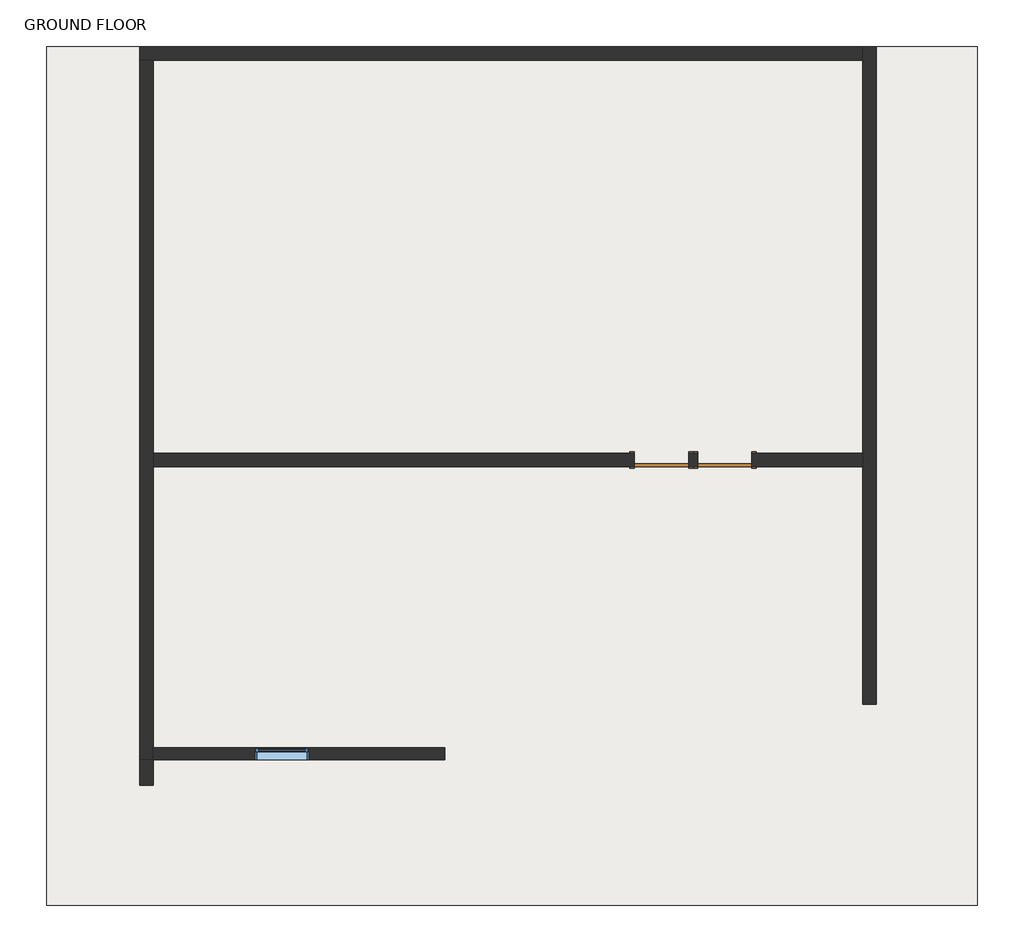
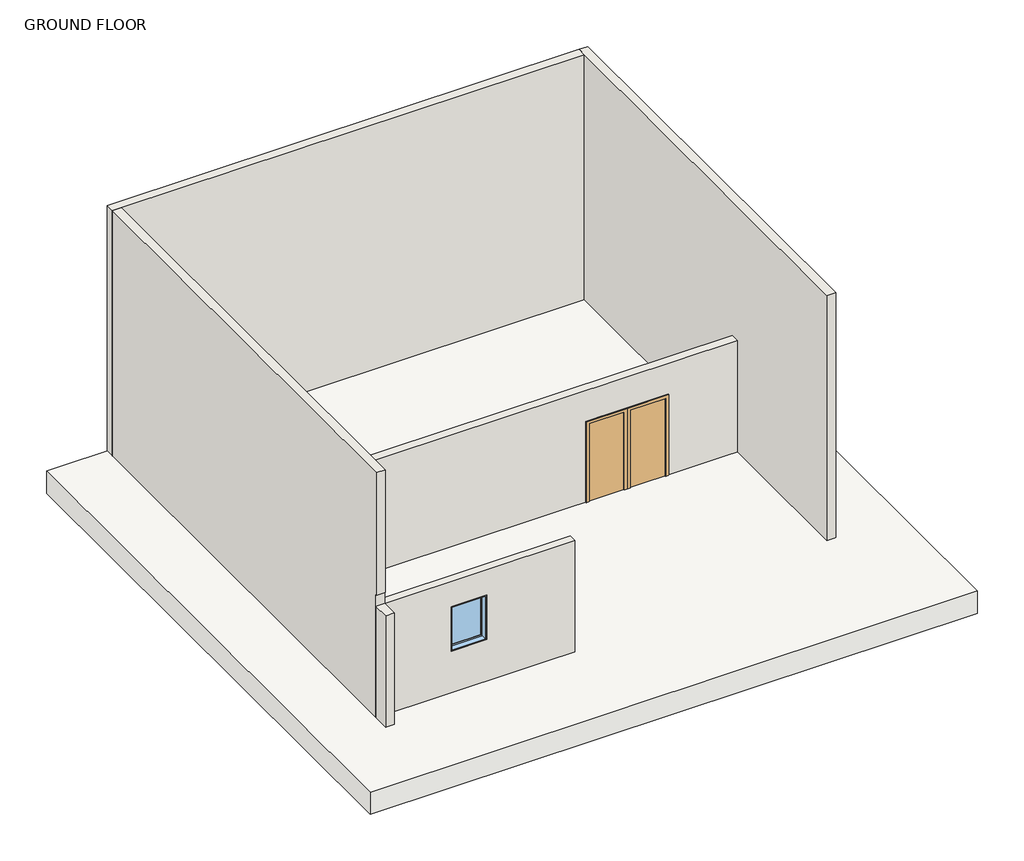
# One storey: 6 walls, 2 doors, 1 slab, 1 window.
"""IFC4 building model written with IfcOpenShell, lengths in millimetres."""

from ifc_helpers import new_model, si_unit, frame, origin, origin_with_axes, place, context, project, spatial, polyline, outline, extrude, faceted_brep, transform, mapped, element, save
from components import door_0ca8825f, window_e2841890

model = new_model("IFC4")

# Units and contexts
model_context = context("Model", 3, world=origin())
ifc_project = project(units=[si_unit("LENGTHUNIT", "METRE", prefix="MILLI")], contexts=[model_context])

# Site, building, storey
site = spatial("IfcSite", under=ifc_project)
building = spatial("IfcBuilding", under=site)
storey = spatial("IfcBuildingStorey", under=building, Name="GROUND FLOOR", Elevation=0.0)

# Doors
placement = place(None, origin())
door_shape = door_0ca8825f(model_context)
element("IfcDoor", 1, ObjectType="Single-Flush : 36\" x 84\"", at=placement, inside=storey, context=model_context, shape_type="MappedRepresentation", body=[
    mapped(door_shape, transform((-4362.8008651, 6476.3047421, 0.0), x_axis=(-1.0, 0.0, 0.0), y_axis=(0.0, -1.0, 0.0), z_axis=(0.0, 0.0, 1.0))),
])
element("IfcDoor", 2, ObjectType="Single-Flush : 36\" x 84\"", at=placement, inside=storey, context=model_context, shape_type="MappedRepresentation", body=[
    mapped(door_shape, transform((-3296.0008651, 6476.3047421, 0.0), x_axis=(-1.0, 0.0, 0.0), y_axis=(0.0, -1.0, 0.0), z_axis=(0.0, 0.0, 1.0))),
])

# Slab
element("IfcSlab", 3, ObjectType="Generic - 12\"", at=placement, inside=storey, context=model_context, shape_type="SweptSolid", body=[
    extrude(outline(polyline([(964.9147214, 13448.6047421), (964.9147214, -1029.3952579), (-14732.2852786, -1029.3952579), (-14732.2852786, 13448.6047421), (964.9147214, 13448.6047421)])), frame((0.0, 0.0, -609.6), z_axis=(0.0, 0.0, 1.0), x_axis=(1.0, 0.0, 0.0)), (0.0, 0.0, 1.0), 609.6),
])

# Walls
element("IfcWall", 4, ObjectType="Generic - 8\"", at=placement, inside=storey, context=model_context, shape_type="SweptSolid", body=[
    extrude(outline(polyline([(0.0, -12935.3008651), (0.0, -8020.4008651), (3048.0, -8020.4008651), (3048.0, -12935.3008651), (0.0, -12935.3008651)]), holes=[polyline([(2353.8279571, -10306.4008651), (1134.6279571, -10306.4008651), (1134.6279571, -11220.8008651), (2353.8279571, -11220.8008651), (2353.8279571, -10306.4008651)])]), frame((0.0, 1421.7047421, 0.0), z_axis=(0.0, 1.0, 0.0), x_axis=(0.0, 0.0, 1.0)), (0.0, 0.0, 1.0), 203.2),
])
element("IfcWall", 5, ObjectType="OTR WALL", at=placement, inside=storey, context=model_context, shape_type="Brep", body=[
    faceted_brep([(-13163.9008651, 13220.0047421, 0.0), (-12935.3008651, 13220.0047421, 0.0), (-971.9008651, 13220.0047421, 0.0), (-971.9008651, 13220.0047421, 6705.6), (-12935.3008651, 13220.0047421, 6705.6), (-13163.9008651, 13220.0047421, 6705.6), (-13163.9008651, 13448.6047421, 0.0), (-13163.9008651, 13448.6047421, 6705.6), (-971.9008651, 13448.6047421, 6705.6), (-971.9008651, 13448.6047421, 0.0)], [[[0, 1, 2, 3, 4, 5]], [[6, 7, 8, 9]], [[2, 1, 0, 6, 9]], [[5, 4, 3, 8, 7]], [[0, 5, 7, 6]], [[3, 2, 9, 8]]]),
])
element("IfcWall", 6, ObjectType="OTR WALL", at=placement, inside=storey, context=model_context, shape_type="Brep", body=[
    faceted_brep([(-12935.3008651, 1421.7047421, 0.0), (-12935.3008651, 1624.9047421, 0.0), (-12935.3008651, 6362.0047421, 0.0), (-12935.3008651, 6590.6047421, 0.0), (-12935.3008651, 13220.0047421, 0.0), (-12935.3008651, 13220.0047421, 6705.6), (-12935.3008651, 6743.0047421, 6705.6), (-12935.3008651, 6514.4047421, 6705.6), (-12935.3008651, 1409.0047421, 6705.6), (-12935.3008651, 1409.0047421, 6400.8), (-12935.3008651, 1409.0047421, 3352.8), (-12935.3008651, 1421.7047421, 3352.8), (-12935.3008651, 1421.7047421, 3048.0), (-13163.9008651, 1421.7047421, 0.0), (-13163.9008651, 1421.7047421, 3048.0), (-13163.9008651, 1421.7047421, 3352.8), (-13163.9008651, 1409.0047421, 3352.8), (-13163.9008651, 1409.0047421, 6400.8), (-13163.9008651, 1409.0047421, 6705.6), (-13163.9008651, 13220.0047421, 6705.6), (-13163.9008651, 13220.0047421, 0.0)], [[[0, 1, 2, 3, 4, 5, 6, 7, 8, 9, 10, 11, 12]], [[13, 14, 15, 16, 17, 18, 19, 20]], [[4, 3, 2, 1, 0, 13, 20]], [[8, 7, 6, 5, 19, 18]], [[5, 4, 20, 19]], [[10, 16, 15, 11]], [[0, 12, 11, 15, 14, 13]], [[8, 18, 17, 16, 10, 9]]]),
])
element("IfcWall", 7, ObjectType="OTR WALL", at=placement, inside=storey, context=model_context, shape_type="Brep", body=[
    faceted_brep([(-971.9008651, 13448.6047421, 0.0), (-971.9008651, 13220.0047421, 0.0), (-971.9008651, 6590.6047421, 0.0), (-971.9008651, 6362.0047421, 0.0), (-971.9008651, 2361.5047421, 0.0), (-971.9008651, 2361.5047421, 3352.8), (-971.9008651, 2361.5047421, 6400.8), (-971.9008651, 2361.5047421, 6705.6), (-971.9008651, 6514.4047421, 6705.6), (-971.9008651, 6743.0047421, 6705.6), (-971.9008651, 13220.0047421, 6705.6), (-971.9008651, 13448.6047421, 6705.6), (-743.3008651, 13448.6047421, 0.0), (-743.3008651, 13448.6047421, 6705.6), (-743.3008651, 2361.5047421, 6705.6), (-743.3008651, 2361.5047421, 6400.8), (-743.3008651, 2361.5047421, 3352.8), (-743.3008651, 2361.5047421, 0.0)], [[[0, 1, 2, 3, 4, 5, 6, 7, 8, 9, 10, 11]], [[12, 13, 14, 15, 16, 17]], [[4, 3, 2, 1, 0, 12, 17]], [[7, 6, 5, 4, 17, 16, 15, 14]], [[11, 10, 9, 8, 7, 14, 13]], [[0, 11, 13, 12]]]),
])
element("IfcWall", 8, ObjectType="OTR WALL", at=placement, inside=storey, context=model_context, shape_type="SweptSolid", body=[
    extrude(outline(polyline([(0.0, -3905.6008651), (0.0, -3753.2008651), (2133.6, -3753.2008651), (2133.6, -2838.8008651), (0.0, -2838.8008651), (0.0, -971.9008651), (3048.0, -971.9008651), (3048.0, -12935.3008651), (0.0, -12935.3008651), (0.0, -4820.0008651), (2133.6, -4820.0008651), (2133.6, -3905.6008651), (0.0, -3905.6008651)])), frame((0.0, 6362.0047421, 0.0), z_axis=(0.0, 1.0, 0.0), x_axis=(0.0, 0.0, 1.0)), (0.0, 0.0, 1.0), 228.6),
])
element("IfcWall", 9, ObjectType="OTR WALL", at=placement, inside=storey, context=model_context, shape_type="SweptSolid", body=[
    extrude(outline(polyline([(-13163.9008651, 989.9047421), (-13163.9008651, 1421.7047421), (-12935.3008651, 1421.7047421), (-12935.3008651, 989.9047421), (-13163.9008651, 989.9047421)])), origin_with_axes(), (0.0, 0.0, 1.0), 3048.0),
])

# Window
window_shape = window_e2841890(model_context)
element("IfcWindow", 10, ObjectType="Fixed : 36\" x 48\"", at=placement, inside=storey, context=model_context, shape_type="MappedRepresentation", body=[
    mapped(window_shape, transform((-10725.5008651, 1523.3047421, 220.2279571), x_axis=(1.0, 0.0, 0.0), y_axis=(0.0, 1.0, 0.0), z_axis=(0.0, 0.0, 1.0))),
])

save(model, "model.ifc")

# Revit data of these elements
# Type "Single-Flush : 36\" x 84\""
#   Type Mark = "1"
#   Construction Type Id = "MDOOR"
#   Assembly Code = "C1020"
#   Analytic Construction = "Metal"
#   Thickness = 0' - 2"
#   Heat Transfer Coefficient (U) = 0.651978 BTU/(h·ft²·°F)
#   Height = 7' - 0"
#   Trim Projection Ext = 0' - 1"
#   Trim Projection Int = 0' - 1"
#   Trim Width = 0' - 3"
#   Width = 3' - 0"
#   Define Thermal Properties by = 1
#   Door Material = Door - Panel
#   Frame Material = Door - Frame
#   Visual Light Transmittance = 0
#   Solar Heat Gain Coefficient = 0
#   Function = (empty or 0)
#   Wall Closure = (empty or 0)
# Type "Generic - 12\""
#   Assembly Code = "B1010"
#   Function = 0
#   Layers, outside or top first: 2' - 0" "Gypsum Wall Board" (function 1)
# Type "Generic - 8\""
#   Assembly Code = "B2010"
#   Layers, outside or top first: 0' - 8" "Default New Material(1)" (function 1)
# Type "OTR WALL"
#   Assembly Code = "B2010"
#   Layers, outside or top first: 0' - 9" "WHITE" (function 1)
# Type "Fixed : 36\" x 48\""
#   Type Mark = "1"
#   Construction Type Id = "GSP4R"
#   Assembly Code = "B2020100"
#   Analytic Construction = "1/8 in Pilkington single glazing"
#   Visual Light Transmittance = 0.9
#   Solar Heat Gain Coefficient = 0.78
#   Heat Transfer Coefficient (U) = 0.6496 BTU/(h·ft²·°F)
#   Height = 4' - 0"
#   Default Sill Height = 3' - 0"
#   Width = 3' - 0"
#   Window Inset = 0' - 0 3/4"
#   Define Thermal Properties by = 1
#   Glass Pane Material = Glass
#   Sash Material = Sash
#   Wall Closure = (empty or 0)
# Elements 1, 2 (IfcDoor, "Single-Flush : 36\" x 84\"")
#   Phase Created = New Construction
#   Materials on its faces: "Door - Frame", "Door - Panel"
# Element 3 (IfcSlab, "Generic - 12\"")
#   Height Offset From Level = 0' - 0"
#   Phase Created = New Construction
#   Materials on its faces: "Gypsum Wall Board"
# Element 4 (IfcWall, "Generic - 8\"")
#   Top Offset = 0' - 0"
#   Base Offset = 0' - 0"
#   Unconnected Height = 10' - 0"
#   wall height = 10' - 0"
#   Phase Created = New Construction
#   Base Constraint = GROUND FLOOR
#   Materials on its faces: "Default New Material(1)"
# Elements 5, 7 (IfcWall, "OTR WALL")
#   Top Offset = 0' - 0"
#   Base Offset = 0' - 0"
#   Unconnected Height = 22' - 0"
#   wall height = 22' - 0"
#   Phase Created = New Construction
#   Base Constraint = GROUND FLOOR
#   Materials on its faces: "WHITE"
# Element 6 (IfcWall, "OTR WALL")
#   Top Offset = 0' - 0"
#   Base Offset = 0' - 0"
#   Unconnected Height = 22' - 0"
#   wall height = 22' - 0"
#   Phase Created = New Construction
#   Base Constraint = GROUND FLOOR
#   Materials on its faces: "WHITE", "Default New Material(1)"
# Elements 8, 9 (IfcWall, "OTR WALL")
#   Top Offset = 0' - 0"
#   Base Offset = 0' - 0"
#   Unconnected Height = 10' - 0"
#   wall height = 10' - 0"
#   Phase Created = New Construction
#   Base Constraint = GROUND FLOOR
#   Materials on its faces: "WHITE"
# Element 10 (IfcWindow, "Fixed : 36\" x 48\"")
#   Mark = "1"
#   Phase Created = New Construction
#   Materials on its faces: "Sash", "Glass"
# Materials
#   "Door - Panel": class "Wood", colour RGB 210 159 95, transparency 0
#   "Door - Frame": colour RGB 118 70 51, transparency 0
#   "Gypsum Wall Board": class "Generic", colour RGB 127 127 127, transparency 0, Description = "Gypsum Wall Board", Cost = 0
#   "Default New Material(1)": class "Generic", colour RGB 192 192 192, transparency 0, Cost = 0
#   "WHITE": class "Generic", colour RGB 255 255 255, transparency 0, Cost = 0
#   "Glass": class "Glass", colour RGB 0 128 192, transparency 0.75, Description = "Soda Lime Glass", Cost = 0
#   "Sash": class "Wood", colour RGB 224 178 126, transparency 0
